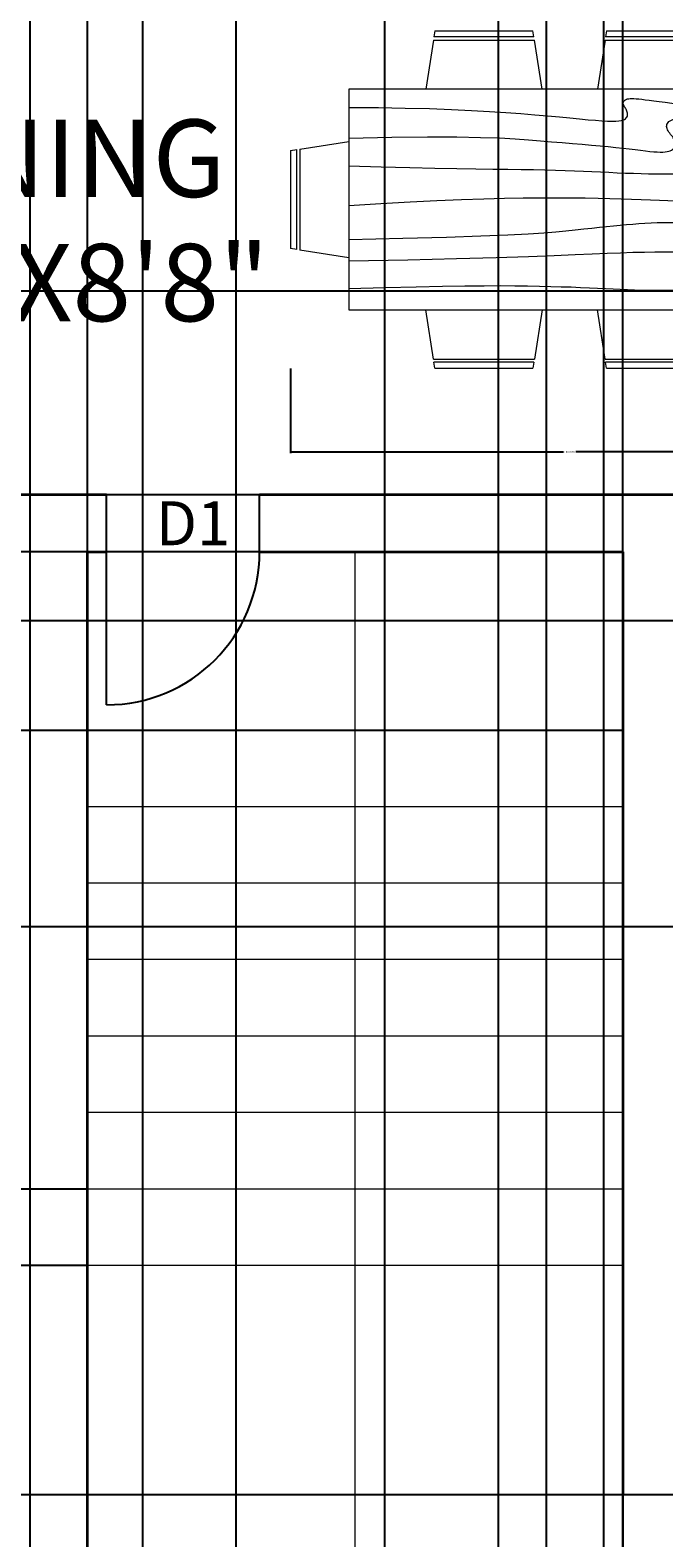
# Model space of a CAD drawing. Units: feet. Extents: x 2270 to 3094, y 1543 to 2352.
# Tile 3 of 6: x 2563 to 2662, y 1813 to 2050. Entities that reach past the tile are written whole.
import ezdxf

# ---------------------------------------------------------------- set-up
doc = ezdxf.new("R2010")
doc.units = ezdxf.units.FT
for name, color, linetype, lineweight in [('A-ANNO-DIMS', 2, 'Continuous', 18), ('A-ANNO-TEXT', 7, 'Continuous', 18), ('A-AREA-IDEN', 7, 'Continuous', 18), ('A-DOOR', 3, 'Continuous', 25), ('A-FLOR-STRS', 7, 'Continuous', 18), ('A-FURN', 8, 'Continuous', 18), ('A-WALL', 7, 'Continuous', 35)]:
    doc.layers.add(name, color=color, linetype=linetype, lineweight=lineweight)
doc.styles.get("Standard").update_dxf_attribs({"font": 'arial.ttf'})
doc.dimstyles.get("Standard").update_dxf_attribs({"dimtxt": 0.18, "dimasz": 0.18, "dimexe": 0.18, "dimexo": 0.0625, "dimgap": 0.09, "dimtad": 0, "dimtih": 1, "dimtoh": 1, "dimdec": 4, "dimzin": 0, "dimdsep": 46, "dimtxsty": 'Standard', "dimcen": 0.09, "dimadec": 0, "dimazin": 0, "dimtfac": 1, "dimtdec": 4, "dimtofl": 0, "dimtmove": 0, "dimatfit": 3, "dimfxl": 1, "dimtolj": 1, "dimtzin": 0, "dimarcsym": 0})

# ---------------------------------------------------------------- blocks, each defined once
blk = doc.blocks.new('Dining Set - 36 x 72 in.')
for p, q in [((-22, 27.5), (-22.1562, 26.50042)), ((-22, 27.5), (-6, 27.5)), ((-5.8437, 26.49966), (-6, 27.5)), ((6, 27.5), (5.8438, 26.50042)), ((6, 27.5), (22, 27.5)), ((22.1563, 26.49966), (22, 27.5)), ((-22.2343, 26.00059), (-23.4847, 17.99762)), ((-22.2304, 26), (-5.7608, 26)), ((-5.8416, 26.5), (-22.1534, 26.5)), ((-4.5152, 17.99762), (-5.7655, 25.99926)), ((5.7657, 26.00059), (4.5153, 17.99762)), ((5.7696, 26), (22.2392, 26)), ((22.1584, 26.5), (5.8466, 26.5)), ((23.4848, 17.99762), (22.2345, 25.99926)), ((36, 18), (-36, 18)), ((-36, 18), (-36, -18)), ((36, -18), (36, 18)), ((-45.5, 8), (-44.5004, 8.15617)), ((-45.5, 8), (-45.5, -8)), ((-44.5, -8.15843), (-44.5, 8.15338)), ((-44.0006, 8.23428), (-35.9976, 9.48474)), ((-44, 8.23041), (-44, -8.23915)), ((44.0006, 8.23428), (35.9976, 9.48474)), ((44, 8.23041), (44, -8.23915)), ((44.5, -8.15843), (44.5, 8.15338)), ((45.5, 8), (44.5005, 8.15617)), ((45.5, 8), (45.5, -8)), ((-44.4997, -8.15631), (-45.5, -8)), ((-35.9976, -9.48476), (-43.9993, -8.2345)), ((35.9976, -9.48476), (43.9993, -8.2345)), ((44.4997, -8.15631), (45.5, -8)), ((-36, -18), (36, -18)), ((-22.2343, -26.0006), (-23.4847, -17.99762)), ((-4.5152, -17.99762), (-5.7655, -25.99928)), ((5.7657, -26.0006), (4.5153, -17.99762)), ((23.4848, -17.99762), (22.2345, -25.99928)), ((-22.2304, -26), (-5.7608, -26)), ((-22, -27.5), (-22.1562, -26.50044)), ((-5.8416, -26.5), (-22.1534, -26.5)), ((-5.8437, -26.49967), (-6, -27.5)), ((5.7696, -26), (22.2392, -26)), ((6, -27.5), (5.8438, -26.50044)), ((22.1584, -26.5), (5.8466, -26.5)), ((22.1563, -26.49967), (22, -27.5)), ((-22, -27.5), (-6, -27.5)), ((6, -27.5), (22, -27.5))]:
    blk.add_line(p, q)
for points in [[(-36, 15), (-31.1772, 14.97754), (-26.8079, 14.91406), (-22.8538, 14.81543), (-19.276, 14.6875), (-16.0362, 14.53613), (-13.0957, 14.36718), (-10.4159, 14.18652), (-7.9583, 14), (-5.6904, 13.81315), (-3.6035, 13.63021), (-1.6954, 13.45508), (0.0365, 13.29166), (1.5945, 13.14388), (2.9811, 13.01562), (4.1988, 12.9108), (5.25, 12.83333), (6.1393, 12.78613), (6.8802, 12.76823), (7.4883, 12.77767), (7.9792, 12.8125), (8.3685, 12.87077), (8.6719, 12.95052), (8.9049, 13.0498), (9.0833, 13.16666), (9.2205, 13.29899), (9.3216, 13.44401), (9.3895, 13.59879), (9.4271, 13.76041), (9.4373, 13.92594), (9.4232, 14.09245), (9.3875, 14.257), (9.3333, 14.41666), (9.2638, 14.56917), (9.1836, 14.71484), (9.0975, 14.85465), (9.0104, 14.98958), (8.9272, 15.1206), (8.8529, 15.2487), (8.7922, 15.37483), (8.75, 15.5), (8.7305, 15.62467), (8.7344, 15.74739), (8.7617, 15.86621), (8.8125, 15.97916), (8.8867, 16.08431), (8.9844, 16.17968), (9.1055, 16.26334), (9.25, 16.33333), (9.4189, 16.38802), (9.6172, 16.42708), (9.8506, 16.45052), (10.125, 16.45833), (10.4463, 16.45052), (10.8203, 16.42708), (11.2529, 16.38802), (11.75, 16.33333), (12.3184, 16.26318), (12.9694, 16.17838), (13.7151, 16.07991), (14.5677, 15.96875), (15.5395, 15.84586), (16.6426, 15.71224), (17.8893, 15.56884), (19.2917, 15.41666), (20.859, 15.25667), (22.5879, 15.08984), (24.4721, 14.91715), (26.5052, 14.73958), (28.6809, 14.5581), (30.9929, 14.3737), (33.4347, 14.18733), (36, 14)], [(-36, 10), (-28.9766, 10.14274), (-23.1725, 10.20442), (-18.4241, 10.19775), (-14.5677, 10.13541), (-11.4399, 10.03011), (-8.877, 9.89453), (-6.7154, 9.74137), (-4.7917, 9.58333), (-2.9698, 9.43082), (-1.2246, 9.28515), (0.4415, 9.14534), (2.026, 9.01041), (3.5266, 8.87939), (4.9408, 8.7513), (6.266, 8.62516), (7.5, 8.5), (8.6411, 8.37549), (9.6914, 8.2539), (10.6538, 8.13818), (11.5312, 8.03125), (12.3267, 7.93603), (13.043, 7.85547), (13.6831, 7.79248), (14.25, 7.75), (14.7471, 7.7303), (15.1797, 7.73307), (15.5537, 7.75732), (15.875, 7.80208), (16.1494, 7.86637), (16.3828, 7.94922), (16.5811, 8.04964), (16.75, 8.16666), (16.8944, 8.29915), (17.0143, 8.44531), (17.1089, 8.60319), (17.1771, 8.77083), (17.218, 8.94629), (17.2305, 9.1276), (17.2137, 9.31282), (17.1667, 9.5), (17.0895, 9.6875), (16.987, 9.875), (16.8649, 10.0625), (16.7292, 10.25), (16.5856, 10.4375), (16.4401, 10.625), (16.2985, 10.8125), (16.1667, 11), (16.05, 11.18733), (15.9518, 11.3737), (15.8752, 11.5581), (15.8229, 11.73958), (15.798, 11.91715), (15.8034, 12.08984), (15.842, 12.25667), (15.9167, 12.41666), (16.0295, 12.56836), (16.1784, 12.70833), (16.3605, 12.83268), (16.5729, 12.9375), (16.8127, 13.01888), (17.0768, 13.07291), (17.3625, 13.0957), (17.6667, 13.08333), (17.9894, 13.03312), (18.3418, 12.94726), (18.7382, 12.82918), (19.1927, 12.68229), (19.7195, 12.51001), (20.3327, 12.31575), (21.0465, 12.10294), (21.875, 11.875), (22.8357, 11.63354), (23.959, 11.37304), (25.2786, 11.08618), (26.8282, 10.76562), (28.6414, 10.40405), (30.752, 9.99414), (33.1936, 9.52856), (36, 9)], [(-36, 5.5), (-30.7157, 5.3348), (-26.069, 5.20963), (-21.9946, 5.11767), (-18.4271, 5.05208), (-15.3009, 5.00602), (-12.5508, 4.97265), (-10.1112, 4.94515), (-7.9167, 4.91666), (-5.909, 4.88167), (-4.0586, 4.83984), (-2.3429, 4.79215), (-0.7396, 4.73958), (0.7739, 4.6831), (2.22, 4.6237), (3.6213, 4.56233), (5, 4.5), (6.373, 4.43782), (7.7344, 4.3776), (9.0723, 4.32129), (10.375, 4.27083), (11.6309, 4.22819), (12.8281, 4.19531), (13.9551, 4.17415), (15, 4.16666), (15.954, 4.17448), (16.819, 4.19791), (17.6001, 4.23698), (18.3021, 4.29166), (18.9299, 4.36198), (19.4883, 4.44791), (19.9823, 4.54948), (20.4167, 4.66666), (20.7969, 4.79899), (21.1302, 4.94401), (21.4245, 5.09879), (21.6875, 5.26041), (21.9271, 5.42594), (22.1511, 5.59245), (22.3672, 5.757), (22.5834, 5.91666), (22.8065, 6.06868), (23.0404, 6.21093), (23.2879, 6.34147), (23.5521, 6.45833), (23.8358, 6.55957), (24.142, 6.64323), (24.4735, 6.70735), (24.8334, 6.75), (25.2235, 6.76969), (25.642, 6.76692), (26.0858, 6.74267), (26.5521, 6.69791), (27.0379, 6.63362), (27.5404, 6.55078), (28.0565, 6.45036), (28.5834, 6.33333), (29.1242, 6.19987), (29.7071, 6.04687), (30.3661, 5.87044), (31.1354, 5.66666), (32.0493, 5.43164), (33.142, 5.16146), (34.4475, 4.85221), (36, 4.5)], [(-36, -1), (-30.7915, -0.6591), (-26.0195, -0.38216), (-21.6519, -0.16284), (-17.6563, 0.00521), (-14.0005, 0.12833), (-10.6523, 0.21289), (-7.5796, 0.26522), (-4.75, 0.29166), (-2.134, 0.29793), (0.2878, 0.28711), (2.5317, 0.26163), (4.6146, 0.22396), (6.5529, 0.17651), (8.3633, 0.12174), (10.0623, 0.06209), (11.6667, 0), (13.1899, -0.06201), (14.6341, -0.1211), (15.9982, -0.17432), (17.2813, -0.21875), (18.4823, -0.25147), (19.6003, -0.26953), (20.6343, -0.27002), (21.5834, -0.25), (22.4481, -0.20768), (23.2357, -0.14584), (23.9549, -0.06836), (24.6146, 0.02083), (25.2235, 0.11784), (25.7904, 0.21875), (26.3241, 0.31966), (26.8334, 0.41666), (27.3265, 0.50618), (27.8099, 0.58593), (28.2894, 0.65397), (28.7709, 0.70833), (29.2601, 0.74707), (29.763, 0.76823), (30.2855, 0.76985), (30.8334, 0.75), (31.4088, 0.70784), (31.9994, 0.64713), (32.589, 0.57275), (33.1615, 0.48958), (33.7008, 0.4025), (34.1908, 0.3164), (34.6153, 0.23616), (34.9584, 0.16666), (35.2099, 0.11165), (35.3848, 0.07031), (35.504, 0.04069), (35.5886, 0.02083), (35.6594, 0.00879), (35.7377, 0.0026), (35.8442, 0.00032), (36, 0)], [(-36, -6.5), (-27.1843, -6.31267), (-20.084, -6.1263), (-14.469, -5.9419), (-10.1094, -5.76042), (-6.7752, -5.58285), (-4.2363, -5.41016), (-2.2629, -5.24333), (-0.625, -5.08334), (0.8708, -4.93099), (2.2715, -4.78646), (3.5872, -4.64974), (4.8281, -4.52084), (6.0046, -4.39974), (7.127, -4.28646), (8.2053, -4.18099), (9.25, -4.08334), (10.2705, -3.99382), (11.2734, -3.91407), (12.2647, -3.84603), (13.25, -3.79167), (14.2354, -3.75293), (15.2266, -3.73177), (16.2295, -3.73015), (17.25, -3.75), (18.2912, -3.79248), (19.3451, -3.85547), (20.4009, -3.93604), (21.4479, -4.03125), (22.4754, -4.13819), (23.4727, -4.25391), (24.4289, -4.37549), (25.3334, -4.5), (26.1785, -4.62492), (26.9694, -4.74935), (27.7145, -4.87281), (28.4219, -4.99479), (29.1, -5.11483), (29.7572, -5.23242), (30.4016, -5.34709), (31.0417, -5.45834), (31.6837, -5.56437), (32.3262, -5.65821), (32.9658, -5.73153), (33.599, -5.77604), (34.2224, -5.78345), (34.8327, -5.74545), (35.4264, -5.65373), (36, -5.5)], [(-36, -10), (-26.4022, -9.81299), (-18.4675, -9.62891), (-11.9839, -9.45069), (-6.7396, -9.28125), (-2.5226, -9.12354), (0.8789, -8.98047), (3.6769, -8.85498), (6.0833, -8.75), (8.2767, -8.66765), (10.3021, -8.60677), (12.1712, -8.56543), (13.8958, -8.54167), (15.4876, -8.53353), (16.9583, -8.53907), (18.3197, -8.55632), (19.5834, -8.58334), (20.7616, -8.61841), (21.8685, -8.66081), (22.9188, -8.71004), (23.9271, -8.76563), (24.9081, -8.82707), (25.8763, -8.89388), (26.8465, -8.96558), (27.8334, -9.04167), (28.8474, -9.12118), (29.8828, -9.20117), (30.93, -9.27824), (31.9792, -9.34896), (33.0205, -9.40991), (34.0443, -9.45768), (35.0407, -9.48885), (36, -9.5)], [(-36, -14.5), (-30.0881, -14.33513), (-25.0332, -14.21224), (-20.7312, -14.12647), (-17.0781, -14.07292), (-13.97, -14.04671), (-11.3027, -14.04297), (-8.9724, -14.05681), (-6.875, -14.08334), (-4.9224, -14.11833), (-3.0905, -14.16016), (-1.3709, -14.20785), (0.2448, -14.26042), (1.7647, -14.3169), (3.1973, -14.3763), (4.5507, -14.43767), (5.8333, -14.5), (7.0554, -14.5621), (8.235, -14.62175), (9.3922, -14.67652), (10.5469, -14.72396), (11.7192, -14.76164), (12.929, -14.78711), (14.1965, -14.79794), (15.5417, -14.79167), (16.9933, -14.76424), (18.6152, -14.70508), (20.4804, -14.60197), (22.6615, -14.44271), (25.2312, -14.21509), (28.2624, -13.9069), (31.8277, -13.50594), (36, -13)]]:
    blk.add_lwpolyline(points)
blk = doc.blocks.new('DOOR-SWING-24')
blk.add_line((33, 0), (0, 0))
blk.add_arc((9, 0), 24, 0, 90)
blk = doc.blocks.new('*D24')
at = {"layer": 'A-ANNO-DIMS', "color": 0, "lineweight": -2, "transparency": 16777216}
for p, q in [((2603.54, 1996.85), (2603.54, 1983.59)), ((2691.16, 1996.85), (2691.16, 1983.59)), ((2603.72, 1983.77), (2646.38, 1983.77)), ((2690.98, 1983.77), (2648.32, 1983.77))]:
    blk.add_line(p, q, dxfattribs=at)
at = {"layer": 'A-ANNO-DIMS', "color": 0, "transparency": 16777216}
for points in [[(2603.72, 1983.8), (2603.72, 1983.74), (2603.54, 1983.77)], [(2690.98, 1983.8), (2690.98, 1983.74), (2691.16, 1983.77)]]:
    blk.add_solid(points, dxfattribs=at)
at = {"layer": 'Defpoints', "color": 0, "transparency": 16777216}
for p in [(2603.54, 1996.92), (2691.16, 1996.92), (2691.16, 1983.77)]:
    blk.add_point(p, dxfattribs=at)
at = {"layer": 'A-ANNO-DIMS', "color": 0, "transparency": 16777216, "insert": (2647.35, 1983.77), "char_height": 0.18, "attachment_point": 5}
blk.add_mtext('\\A1;DINING SET 88', dxfattribs=at)
blk = doc.blocks.new('*D34')
at = {"layer": 'A-ANNO-DIMS', "color": 0, "lineweight": -2, "transparency": 16777216}
for p, q in [((2580.32, 2252.02), (2580.32, 1574.6)), ((2618.3, 2252.02), (2618.3, 1574.6)), ((2580.5, 1574.78), (2598.92, 1574.78)), ((2618.12, 1574.78), (2599.7, 1574.78))]:
    blk.add_line(p, q, dxfattribs=at)
at = {"layer": 'A-ANNO-DIMS', "color": 0, "transparency": 16777216}
for points in [[(2580.5, 1574.81), (2580.5, 1574.75), (2580.32, 1574.78)], [(2618.12, 1574.81), (2618.12, 1574.75), (2618.3, 1574.78)]]:
    blk.add_solid(points, dxfattribs=at)
at = {"layer": 'Defpoints', "color": 0, "transparency": 16777216}
for p in [(2580.32, 2252.08), (2618.3, 2252.08), (2618.3, 1574.78)]:
    blk.add_point(p, dxfattribs=at)
at = {"layer": 'A-ANNO-DIMS', "color": 0, "transparency": 16777216, "insert": (2599.31, 1574.78), "char_height": 0.18, "attachment_point": 5}
blk.add_mtext('\\A1;37.98', dxfattribs=at)
blk = doc.blocks.new('*D35')
at = {"layer": 'A-ANNO-DIMS', "color": 0, "lineweight": -2, "transparency": 16777216}
for p, q in [((2618.3, 2243.02), (2618.3, 1574.6)), ((2643.67, 2243.02), (2643.67, 1574.6)), ((2618.48, 1574.78), (2630.52, 1574.78)), ((2643.49, 1574.78), (2631.45, 1574.78))]:
    blk.add_line(p, q, dxfattribs=at)
at = {"layer": 'A-ANNO-DIMS', "color": 0, "transparency": 16777216}
for points in [[(2618.48, 1574.81), (2618.48, 1574.75), (2618.3, 1574.78)], [(2643.49, 1574.81), (2643.49, 1574.75), (2643.67, 1574.78)]]:
    blk.add_solid(points, dxfattribs=at)
at = {"layer": 'Defpoints', "color": 0, "transparency": 16777216}
for p in [(2618.3, 2243.08), (2643.67, 2243.08), (2643.67, 1574.78)]:
    blk.add_point(p, dxfattribs=at)
at = {"layer": 'A-ANNO-DIMS', "color": 0, "transparency": 16777216, "insert": (2630.98, 1574.78), "char_height": 0.18, "attachment_point": 5}
blk.add_mtext('\\A1;25.366', dxfattribs=at)
blk = doc.blocks.new('*D36')
at = {"layer": 'A-ANNO-DIMS', "color": 0, "lineweight": -2, "transparency": 16777216}
for p, q in [((2652.67, 2243.02), (2652.67, 1574.6)), ((2684.42, 2243.02), (2684.42, 1574.6)), ((2652.85, 1574.78), (2668.15, 1574.78)), ((2684.24, 1574.78), (2668.94, 1574.78))]:
    blk.add_line(p, q, dxfattribs=at)
at = {"layer": 'A-ANNO-DIMS', "color": 0, "transparency": 16777216}
for points in [[(2652.85, 1574.81), (2652.85, 1574.75), (2652.67, 1574.78)], [(2684.24, 1574.81), (2684.24, 1574.75), (2684.42, 1574.78)]]:
    blk.add_solid(points, dxfattribs=at)
at = {"layer": 'Defpoints', "color": 0, "transparency": 16777216}
for p in [(2652.67, 2243.08), (2684.42, 2243.08), (2684.42, 1574.78)]:
    blk.add_point(p, dxfattribs=at)
at = {"layer": 'A-ANNO-DIMS', "color": 0, "transparency": 16777216, "insert": (2668.55, 1574.78), "char_height": 0.18, "attachment_point": 5}
blk.add_mtext('\\A1;31.76', dxfattribs=at)
blk = doc.blocks.new('*D44')
at = {"layer": 'A-ANNO-DIMS', "color": 0, "lineweight": -2, "transparency": 16777216}
for p, q in [((2816.6, 1957.26), (2270.19, 1957.26)), ((2270.37, 1957.08), (2270.37, 1933.44)), ((2270.37, 1909.44), (2270.37, 1933.08)), ((2816.6, 1909.26), (2270.19, 1909.26))]:
    blk.add_line(p, q, dxfattribs=at)
at = {"layer": 'A-ANNO-DIMS', "color": 0, "transparency": 16777216}
for points in [[(2270.34, 1957.08), (2270.4, 1957.08), (2270.37, 1957.26)], [(2270.34, 1909.44), (2270.4, 1909.44), (2270.37, 1909.26)]]:
    blk.add_solid(points, dxfattribs=at)
at = {"layer": 'Defpoints', "color": 0, "transparency": 16777216}
for p in [(2270.37, 1957.26), (2816.67, 1957.26), (2816.67, 1909.26)]:
    blk.add_point(p, dxfattribs=at)
at = {"layer": 'A-ANNO-DIMS', "color": 0, "transparency": 16777216, "insert": (2270.37, 1933.26), "char_height": 0.18, "attachment_point": 5}
blk.add_mtext('\\A1;48', dxfattribs=at)
blk = doc.blocks.new('*D45')
at = {"layer": 'A-ANNO-DIMS', "color": 0, "lineweight": -2, "transparency": 16777216}
for p, q in [((2816.6, 1909.26), (2270.19, 1909.26)), ((2270.37, 1909.08), (2270.37, 1864.85)), ((2270.37, 1820.26), (2270.37, 1864.49)), ((2816.6, 1820.08), (2270.19, 1820.08))]:
    blk.add_line(p, q, dxfattribs=at)
at = {"layer": 'A-ANNO-DIMS', "color": 0, "transparency": 16777216}
for points in [[(2270.34, 1909.08), (2270.4, 1909.08), (2270.37, 1909.26)], [(2270.34, 1820.26), (2270.4, 1820.26), (2270.37, 1820.08)]]:
    blk.add_solid(points, dxfattribs=at)
at = {"layer": 'Defpoints', "color": 0, "transparency": 16777216}
for p in [(2270.37, 1909.26), (2816.67, 1909.26), (2816.67, 1820.08)]:
    blk.add_point(p, dxfattribs=at)
at = {"layer": 'A-ANNO-DIMS', "color": 0, "transparency": 16777216, "insert": (2270.37, 1864.67), "char_height": 0.18, "attachment_point": 5}
blk.add_mtext('\\A1;89.18', dxfattribs=at)
blk = doc.blocks.new('*D52')
at = {"layer": 'A-ANNO-DIMS', "color": 0, "lineweight": -2, "transparency": 16777216}
for p, q in [((2594.98, 1683.15), (2594.98, 2351.56)), ((2595.16, 2351.38), (2615.09, 2351.38)), ((2635.97, 2351.38), (2616.03, 2351.38)), ((2636.15, 1683.15), (2636.15, 2351.56))]:
    blk.add_line(p, q, dxfattribs=at)
at = {"layer": 'A-ANNO-DIMS', "color": 0, "transparency": 16777216}
for points in [[(2595.16, 2351.41), (2595.16, 2351.35), (2594.98, 2351.38)], [(2635.97, 2351.41), (2635.97, 2351.35), (2636.15, 2351.38)]]:
    blk.add_solid(points, dxfattribs=at)
at = {"layer": 'Defpoints', "color": 0, "transparency": 16777216}
for p in [(2636.15, 2351.38), (2594.98, 1683.08), (2636.15, 1683.08)]:
    blk.add_point(p, dxfattribs=at)
at = {"layer": 'A-ANNO-DIMS', "color": 0, "transparency": 16777216, "insert": (2615.56, 2351.38), "char_height": 0.18, "attachment_point": 5}
blk.add_mtext('\\A1;41.175', dxfattribs=at)
blk = doc.blocks.new('*D53')
at = {"layer": 'A-ANNO-DIMS', "color": 0, "lineweight": -2, "transparency": 16777216}
for p, q in [((2636.15, 1683.15), (2636.15, 2351.56)), ((2636.33, 2351.38), (2645.45, 2351.38)), ((2655.49, 2351.38), (2646.36, 2351.38)), ((2655.67, 1683.15), (2655.67, 2351.56))]:
    blk.add_line(p, q, dxfattribs=at)
at = {"layer": 'A-ANNO-DIMS', "color": 0, "transparency": 16777216}
for points in [[(2636.33, 2351.41), (2636.33, 2351.35), (2636.15, 2351.38)], [(2655.49, 2351.41), (2655.49, 2351.35), (2655.67, 2351.38)]]:
    blk.add_solid(points, dxfattribs=at)
at = {"layer": 'Defpoints', "color": 0, "transparency": 16777216}
for p in [(2655.67, 2351.38), (2636.15, 1683.08), (2655.67, 1683.08)]:
    blk.add_point(p, dxfattribs=at)
at = {"layer": 'A-ANNO-DIMS', "color": 0, "transparency": 16777216, "insert": (2645.91, 2351.38), "char_height": 0.18, "attachment_point": 5}
blk.add_mtext('\\A1;19.516', dxfattribs=at)
blk = doc.blocks.new('*D56')
at = {"layer": 'A-ANNO-DIMS', "color": 0, "lineweight": -2, "transparency": 16777216}
for p, q in [((2378.73, 2009.08), (3094.15, 2009.08)), ((3093.97, 2008.9), (3093.97, 1993.27)), ((3093.97, 1977.26), (3093.97, 1992.9)), ((2378.73, 1977.08), (3094.15, 1977.08))]:
    blk.add_line(p, q, dxfattribs=at)
at = {"layer": 'A-ANNO-DIMS', "color": 0, "transparency": 16777216}
for points in [[(3093.94, 2008.9), (3094, 2008.9), (3093.97, 2009.08)], [(3093.94, 1977.26), (3094, 1977.26), (3093.97, 1977.08)]]:
    blk.add_solid(points, dxfattribs=at)
at = {"layer": 'Defpoints', "color": 0, "transparency": 16777216}
for p in [(2378.67, 2009.08), (3093.97, 2009.08), (2378.67, 1977.08)]:
    blk.add_point(p, dxfattribs=at)
at = {"layer": 'A-ANNO-DIMS', "color": 0, "transparency": 16777216, "insert": (3093.97, 1993.08), "char_height": 0.18, "attachment_point": 5}
blk.add_mtext('\\A1;32', dxfattribs=at)
blk = doc.blocks.new('*D61')
at = {"layer": 'A-ANNO-DIMS', "color": 0, "lineweight": -2, "transparency": 16777216}
for p, q in [((2571.67, 1968.02), (2571.67, 1574.6)), ((2655.67, 1968.02), (2655.67, 1574.6)), ((2571.85, 1574.78), (2613.45, 1574.78)), ((2655.49, 1574.78), (2613.88, 1574.78))]:
    blk.add_line(p, q, dxfattribs=at)
at = {"layer": 'A-ANNO-DIMS', "color": 0, "transparency": 16777216}
for points in [[(2571.85, 1574.81), (2571.85, 1574.75), (2571.67, 1574.78)], [(2655.49, 1574.81), (2655.49, 1574.75), (2655.67, 1574.78)]]:
    blk.add_solid(points, dxfattribs=at)
at = {"layer": 'Defpoints', "color": 0, "transparency": 16777216}
for p in [(2571.67, 1968.08), (2655.67, 1968.08), (2655.67, 1574.78)]:
    blk.add_point(p, dxfattribs=at)
at = {"layer": 'A-ANNO-DIMS', "color": 0, "transparency": 16777216, "insert": (2613.67, 1574.78), "char_height": 0.18, "attachment_point": 5}
blk.add_mtext('\\A1;84', dxfattribs=at)
blk = doc.blocks.new('*D62')
at = {"layer": 'A-ANNO-DIMS', "color": 0, "lineweight": -2, "transparency": 16777216}
for p, q in [((2571.6, 1868.08), (2270.19, 1868.08)), ((2270.37, 1867.9), (2270.37, 1862.26)), ((2270.37, 1856.26), (2270.37, 1861.9)), ((2571.6, 1856.08), (2270.19, 1856.08))]:
    blk.add_line(p, q, dxfattribs=at)
at = {"layer": 'A-ANNO-DIMS', "color": 0, "transparency": 16777216}
for points in [[(2270.34, 1867.9), (2270.4, 1867.9), (2270.37, 1868.08)], [(2270.34, 1856.26), (2270.4, 1856.26), (2270.37, 1856.08)]]:
    blk.add_solid(points, dxfattribs=at)
at = {"layer": 'Defpoints', "color": 0, "transparency": 16777216}
for p in [(2270.37, 1868.08), (2571.67, 1868.08), (2571.67, 1856.08)]:
    blk.add_point(p, dxfattribs=at)
at = {"layer": 'A-ANNO-DIMS', "color": 0, "transparency": 16777216, "insert": (2270.37, 1862.08), "char_height": 0.18, "attachment_point": 5}
blk.add_mtext('\\A1;12', dxfattribs=at)
blk = doc.blocks.new('*D63')
at = {"layer": 'A-ANNO-DIMS', "color": 0, "lineweight": -2, "transparency": 16777216}
for p, q in [((2655.6, 1968.08), (2270.19, 1968.08)), ((2270.37, 1967.9), (2270.37, 1954.27)), ((2270.37, 1940.26), (2270.37, 1953.9)), ((2655.6, 1940.08), (2270.19, 1940.08))]:
    blk.add_line(p, q, dxfattribs=at)
at = {"layer": 'A-ANNO-DIMS', "color": 0, "transparency": 16777216}
for points in [[(2270.34, 1967.9), (2270.4, 1967.9), (2270.37, 1968.08)], [(2270.34, 1940.26), (2270.4, 1940.26), (2270.37, 1940.08)]]:
    blk.add_solid(points, dxfattribs=at)
at = {"layer": 'Defpoints', "color": 0, "transparency": 16777216}
for p in [(2270.37, 1968.08), (2655.67, 1968.08), (2655.67, 1940.08)]:
    blk.add_point(p, dxfattribs=at)
at = {"layer": 'A-ANNO-DIMS', "color": 0, "transparency": 16777216, "insert": (2270.37, 1954.08), "char_height": 0.18, "attachment_point": 5}
blk.add_mtext('\\A1;28', dxfattribs=at)
blk = doc.blocks.new('*D65')
at = {"layer": 'A-ANNO-DIMS', "color": 0, "lineweight": -2, "transparency": 16777216}
for p, q in [((2562.67, 1683.15), (2562.67, 2351.56)), ((2562.85, 2351.38), (2567.02, 2351.38)), ((2571.49, 2351.38), (2567.32, 2351.38)), ((2571.67, 1683.15), (2571.67, 2351.56))]:
    blk.add_line(p, q, dxfattribs=at)
at = {"layer": 'A-ANNO-DIMS', "color": 0, "transparency": 16777216}
for points in [[(2562.85, 2351.41), (2562.85, 2351.35), (2562.67, 2351.38)], [(2571.49, 2351.41), (2571.49, 2351.35), (2571.67, 2351.38)]]:
    blk.add_solid(points, dxfattribs=at)
at = {"layer": 'Defpoints', "color": 0, "transparency": 16777216}
for p in [(2571.67, 2351.38), (2562.67, 1683.08), (2571.67, 1683.08)]:
    blk.add_point(p, dxfattribs=at)
at = {"layer": 'A-ANNO-DIMS', "color": 0, "transparency": 16777216, "insert": (2567.17, 2351.38), "char_height": 0.18, "attachment_point": 5}
blk.add_mtext('\\A1;9', dxfattribs=at)

msp = doc.modelspace()

# ---------------------------------------------------------------- linework, layer by layer
at = {"layer": 'A-DOOR'}
msp.add_line((2598.6659, 1968.0845), (2598.6659, 1977.0845), dxfattribs=at)
at = {"layer": 'A-FLOR-STRS'}
for p, q in [((2613.6659, 1811.0845), (2613.6659, 1968.0845)), ((2655.6659, 1940.0845), (2571.6659, 1940.0845)), ((2655.6659, 1928.0845), (2571.6659, 1928.0845)), ((2655.6659, 1916.0845), (2571.6659, 1916.0845)), ((2655.6659, 1904.0845), (2571.6659, 1904.0845)), ((2655.6659, 1892.0845), (2571.6659, 1892.0845)), ((2655.6659, 1880.0845), (2571.6659, 1880.0845)), ((2655.6659, 1868.0845), (2571.6659, 1868.0845)), ((2655.6659, 1856.0845), (2571.6659, 1856.0845)), ((2655.6659, 1820.0845), (2613.6659, 1820.0845))]:
    msp.add_line(p, q, dxfattribs=at)
at = {"layer": 'A-WALL'}
for p, q in [((2559.6659, 1977.0845), (2574.6659, 1977.0845)), ((2571.6659, 1977.0845), (2574.6659, 1977.0845)), ((2598.6659, 1977.0845), (2724.8399, 1977.0845)), ((2598.6659, 1977.0845), (2655.6659, 1977.0845)), ((2571.6659, 1968.0845), (2574.6659, 1968.0845)), ((2571.6659, 1804.0845), (2571.6659, 1968.0845)), ((2598.6659, 1968.0845), (2655.6659, 1968.0845)), ((2655.6659, 1968.0845), (2655.6659, 1820.0845))]:
    msp.add_line(p, q, dxfattribs=at)

# ---------------------------------------------------------------- block references
at = {"layer": 'A-DOOR', "rotation": 269.9999999999994}
msp.add_blockref('DOOR-SWING-24', (2574.6664, 1977.0844), dxfattribs=at)
at = {"layer": 'A-FURN', "xscale": 0.96282654590751, "yscale": 0.96282654590751, "zscale": 0.96282654590751}
msp.add_blockref('Dining Set - 36 x 72 in.', (2647.3519, 2023.3951), dxfattribs=at)

# ---------------------------------------------------------------- texts
at = {"layer": 'A-ANNO-TEXT'}
msp.add_text('D1', height=6.89564, dxfattribs=at).set_placement((2582.3841, 1969.1303))
at = {"layer": 'A-AREA-IDEN'}
for s, p in [('DINING', (2536.8128, 2023.7996)), ('18\'X8\'8"', (2536.8128, 2004.2888))]:
    msp.add_text(s, height=12.14556, dxfattribs=at).set_placement(p)

# ---------------------------------------------------------------- dimensions: what is measured, and where the dimension line sits
at = {"layer": 'A-ANNO-DIMS'}
for base, p1, p2, override, picture, middle in [((2571.6659, 2351.3845), (2562.6659, 1683.0845), (2571.6659, 1683.0845), {"dimdec": 0, "dimlfac": 1, "dimrnd": 0, "dimzin": 0, "dimdsep": 46, "dimlunit": 2}, '*D65', (2567.1659, 2351.3845)), ((2636.1502, 2351.3845), (2594.9751, 1683.0845), (2636.1502, 1683.0845), {"dimdec": 3, "dimlfac": 1, "dimrnd": 0, "dimzin": 0, "dimdsep": 46, "dimlunit": 2}, '*D52', (2615.5626, 2351.3845)), ((2655.6659, 2351.3845), (2636.1502, 1683.0845), (2655.6659, 1683.0845), {"dimdec": 3, "dimlfac": 1, "dimrnd": 0, "dimzin": 0, "dimdsep": 46, "dimlunit": 2}, '*D53', (2645.9081, 2351.3845)), ((2618.2997, 1574.7845), (2580.3205, 2252.0845), (2618.2997, 2252.0845), {"dimdec": 2, "dimlfac": 1, "dimrnd": 0, "dimzin": 0, "dimdsep": 46, "dimlunit": 2}, '*D34', (2599.3101, 1574.7845)), ((2643.6659, 1574.7845), (2618.2997, 2243.0845), (2643.6659, 2243.0845), {"dimdec": 3, "dimlfac": 1, "dimrnd": 0, "dimzin": 0, "dimdsep": 46, "dimlunit": 2}, '*D35', (2630.9828, 1574.7845)), ((2684.4243, 1574.7845), (2652.6659, 2243.0845), (2684.4243, 2243.0845), {"dimdec": 2, "dimlfac": 1, "dimrnd": 0, "dimzin": 0, "dimdsep": 46, "dimlunit": 2}, '*D36', (2668.5451, 1574.7845)), ((2655.6659, 1574.7845), (2571.6659, 1968.0845), (2655.6659, 1968.0845), {"dimdec": 0, "dimlfac": 1, "dimrnd": 0, "dimzin": 0, "dimdsep": 46, "dimlunit": 2}, '*D61', (2613.6659, 1574.7845))]:
    dim = msp.add_linear_dim(base=base, p1=p1, p2=p2, dimstyle='Standard', override=override, dxfattribs=at)
    dim.commit()
    dim.dimension.update_dxf_attribs({"geometry": picture, "text_midpoint": middle})
for base, p1, p2, override, picture, middle in [((3093.9659, 2009.0845), (2378.6659, 1977.0845), (2378.6659, 2009.0845), {"dimdec": 0, "dimlfac": 1, "dimrnd": 0, "dimzin": 0, "dimdsep": 46, "dimlunit": 2}, '*D56', (3093.9659, 1993.0845)), ((2270.3659, 1968.0845), (2655.6659, 1940.0845), (2655.6659, 1968.0845), {"dimdec": 0, "dimlfac": 1, "dimrnd": 0, "dimzin": 0, "dimdsep": 46, "dimlunit": 2}, '*D63', (2270.3659, 1954.0845)), ((2270.3659, 1957.2599), (2816.6659, 1909.2599), (2816.6659, 1957.2599), {"dimdec": 0, "dimlfac": 1, "dimrnd": 0, "dimzin": 0, "dimdsep": 46, "dimlunit": 2}, '*D44', (2270.3659, 1933.2599)), ((2270.3659, 1909.2599), (2816.6659, 1820.0845), (2816.6659, 1909.2599), {"dimdec": 2, "dimlfac": 1, "dimrnd": 0, "dimzin": 0, "dimdsep": 46, "dimlunit": 2}, '*D45', (2270.3659, 1864.6722)), ((2270.3659, 1868.0845), (2571.6659, 1856.0845), (2571.6659, 1868.0845), {"dimdec": 0, "dimlfac": 1, "dimrnd": 0, "dimzin": 0, "dimdsep": 46, "dimlunit": 2}, '*D62', (2270.3659, 1862.0845))]:
    dim = msp.add_linear_dim(base=base, p1=p1, p2=p2, angle=90, dimstyle='Standard', override=override, dxfattribs=at)
    dim.commit()
    dim.dimension.update_dxf_attribs({"geometry": picture, "text_midpoint": middle})
dim = msp.add_linear_dim(base=(2691.1605, 1983.7748), p1=(2603.5433, 1996.9174), p2=(2691.1605, 1996.9174), text='DINING SET <>', dimstyle='Standard', override={"dimdec": 0, "dimlfac": 1, "dimrnd": 0, "dimzin": 0, "dimdsep": 46, "dimlunit": 2}, dxfattribs=at)
dim.commit()
dim.dimension.update_dxf_attribs({"geometry": '*D24', "text_midpoint": (2647.3519, 1983.7748)})

doc.saveas('drawing.dxf')
